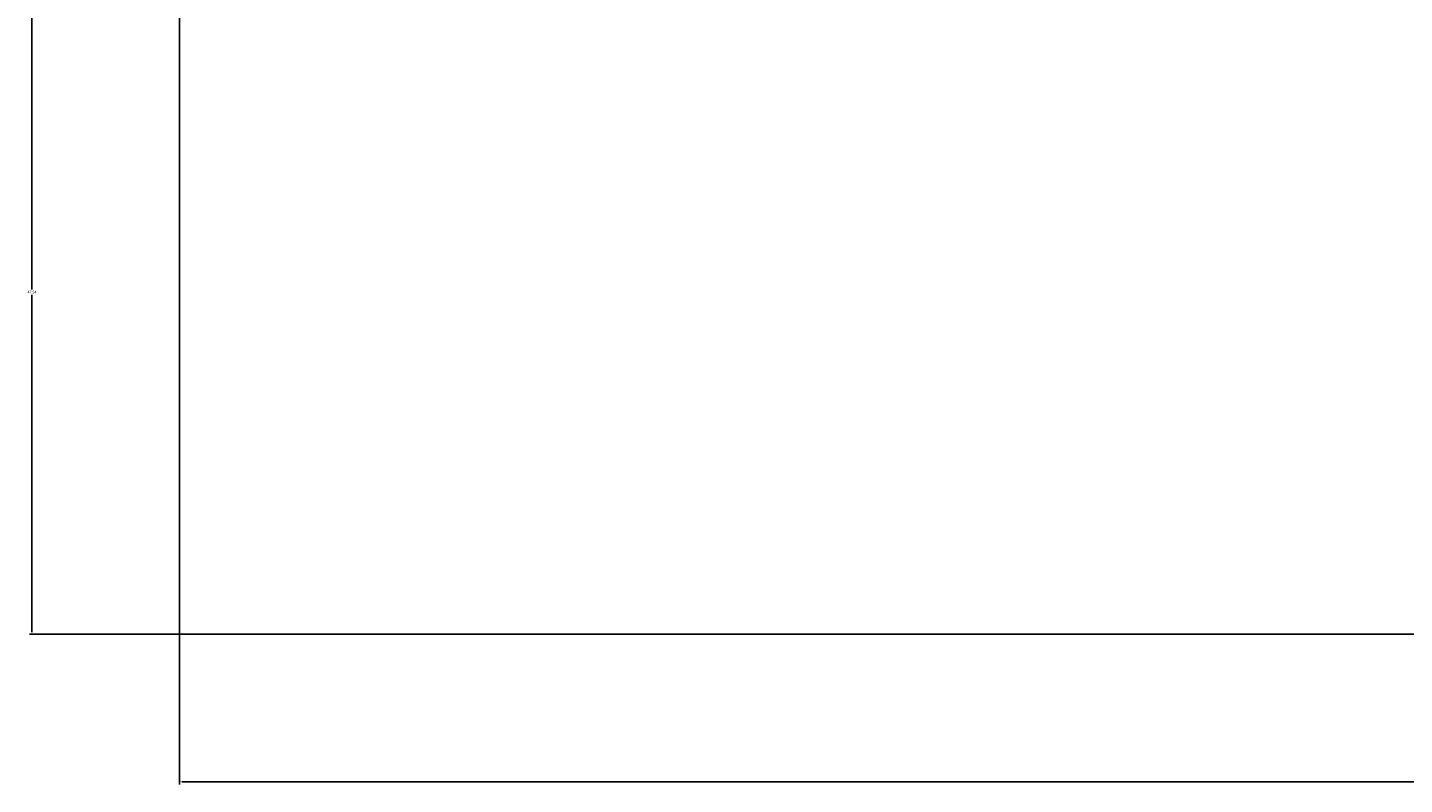
# Model space of a CAD drawing. Units: millimetres. Extents: x 446512 to 447461, y 70395 to 70610.
# Tile 28 of 39: x 447244 to 447340, y 70395 to 70447. Entities that reach past the tile are written whole.
import ezdxf

# ---------------------------------------------------------------- set-up
doc = ezdxf.new("R2010")
doc.units = ezdxf.units.MM
doc.layers.add('A-ANNO-DIMS', color=2, linetype='Continuous', lineweight=18)
doc.styles.get("Standard").update_dxf_attribs({"font": 'arial.ttf'})
doc.dimstyles.get("Standard").update_dxf_attribs({"dimtxt": 0.18, "dimasz": 0.18, "dimexe": 0.18, "dimexo": 0.0625, "dimgap": 0.09, "dimtad": 0, "dimtih": 1, "dimtoh": 1, "dimdec": 4, "dimzin": 0, "dimdsep": 46, "dimtxsty": 'Standard', "dimcen": 0.09, "dimadec": 0, "dimazin": 0, "dimtfac": 1, "dimtdec": 4, "dimtofl": 0, "dimtmove": 0, "dimatfit": 3, "dimfxl": 1, "dimtolj": 1, "dimtzin": 0, "dimarcsym": 0})

# ---------------------------------------------------------------- blocks, each defined once
blk = doc.blocks.new('*D61')
at = {"layer": 'A-ANNO-DIMS', "color": 0, "lineweight": -2, "transparency": 16777216}
for p, q in [((447254.943, 70452.792), (447254.943, 70394.885)), ((447450.532, 70432.19), (447450.532, 70394.885)), ((447255.123, 70395.065), (447352.352, 70395.065)), ((447450.352, 70395.065), (447353.122, 70395.065))]:
    blk.add_line(p, q, dxfattribs=at)
at = {"layer": 'A-ANNO-DIMS', "color": 0, "transparency": 16777216}
for points in [[(447255.123, 70395.095), (447255.123, 70395.035), (447254.943, 70395.065)], [(447450.352, 70395.095), (447450.352, 70395.035), (447450.532, 70395.065)]]:
    blk.add_solid(points, dxfattribs=at)
at = {"layer": 'Defpoints', "color": 0, "transparency": 16777216}
for p in [(447254.943, 70452.855), (447450.532, 70432.253), (447450.532, 70395.065)]:
    blk.add_point(p, dxfattribs=at)
at = {"layer": 'A-ANNO-DIMS', "color": 0, "transparency": 16777216, "insert": (447352.737, 70395.065), "char_height": 0.18, "attachment_point": 5}
blk.add_mtext('\\A1;195.6', dxfattribs=at)
blk = doc.blocks.new('*D72')
at = {"layer": 'A-ANNO-DIMS', "color": 0, "lineweight": -2, "transparency": 16777216}
for p, q in [((447254.88, 70452.855), (447244.513, 70452.855)), ((447244.693, 70452.675), (447244.693, 70429.266)), ((447244.693, 70405.495), (447244.693, 70428.903)), ((447365.363, 70405.315), (447244.513, 70405.315))]:
    blk.add_line(p, q, dxfattribs=at)
at = {"layer": 'A-ANNO-DIMS', "color": 0, "transparency": 16777216}
for points in [[(447244.663, 70452.675), (447244.723, 70452.675), (447244.693, 70452.855)], [(447244.663, 70405.495), (447244.723, 70405.495), (447244.693, 70405.315)]]:
    blk.add_solid(points, dxfattribs=at)
at = {"layer": 'Defpoints', "color": 0, "transparency": 16777216}
for p in [(447244.693, 70452.855), (447254.943, 70452.855), (447365.425, 70405.315)]:
    blk.add_point(p, dxfattribs=at)
at = {"layer": 'A-ANNO-DIMS', "color": 0, "transparency": 16777216, "insert": (447244.693, 70429.085), "char_height": 0.18, "attachment_point": 5}
blk.add_mtext('\\A1;47.54', dxfattribs=at)

msp = doc.modelspace()

# ---------------------------------------------------------------- dimensions: what is measured, and where the dimension line sits
at = {"layer": 'A-ANNO-DIMS'}
dim = msp.add_linear_dim(base=(447244.6927, 70452.855), p1=(447365.4251, 70405.3145), p2=(447254.9427, 70452.855), angle=90, dimstyle='Standard', override={"dimdec": 2, "dimlfac": 1, "dimrnd": 0, "dimzin": 0, "dimdsep": 46, "dimlunit": 2}, dxfattribs=at)
dim.commit()
dim.dimension.update_dxf_attribs({"geometry": '*D72', "text_midpoint": (447244.6927, 70429.0848)})
dim = msp.add_linear_dim(base=(447450.5318, 70395.0645), p1=(447254.9427, 70452.855), p2=(447450.5318, 70432.2526), dimstyle='Standard', override={"dimdec": 1, "dimlfac": 1, "dimrnd": 0, "dimzin": 0, "dimdsep": 46, "dimlunit": 2}, dxfattribs=at)
dim.commit()
dim.dimension.update_dxf_attribs({"geometry": '*D61', "text_midpoint": (447352.7372, 70395.0645)})

doc.saveas('drawing.dxf')
